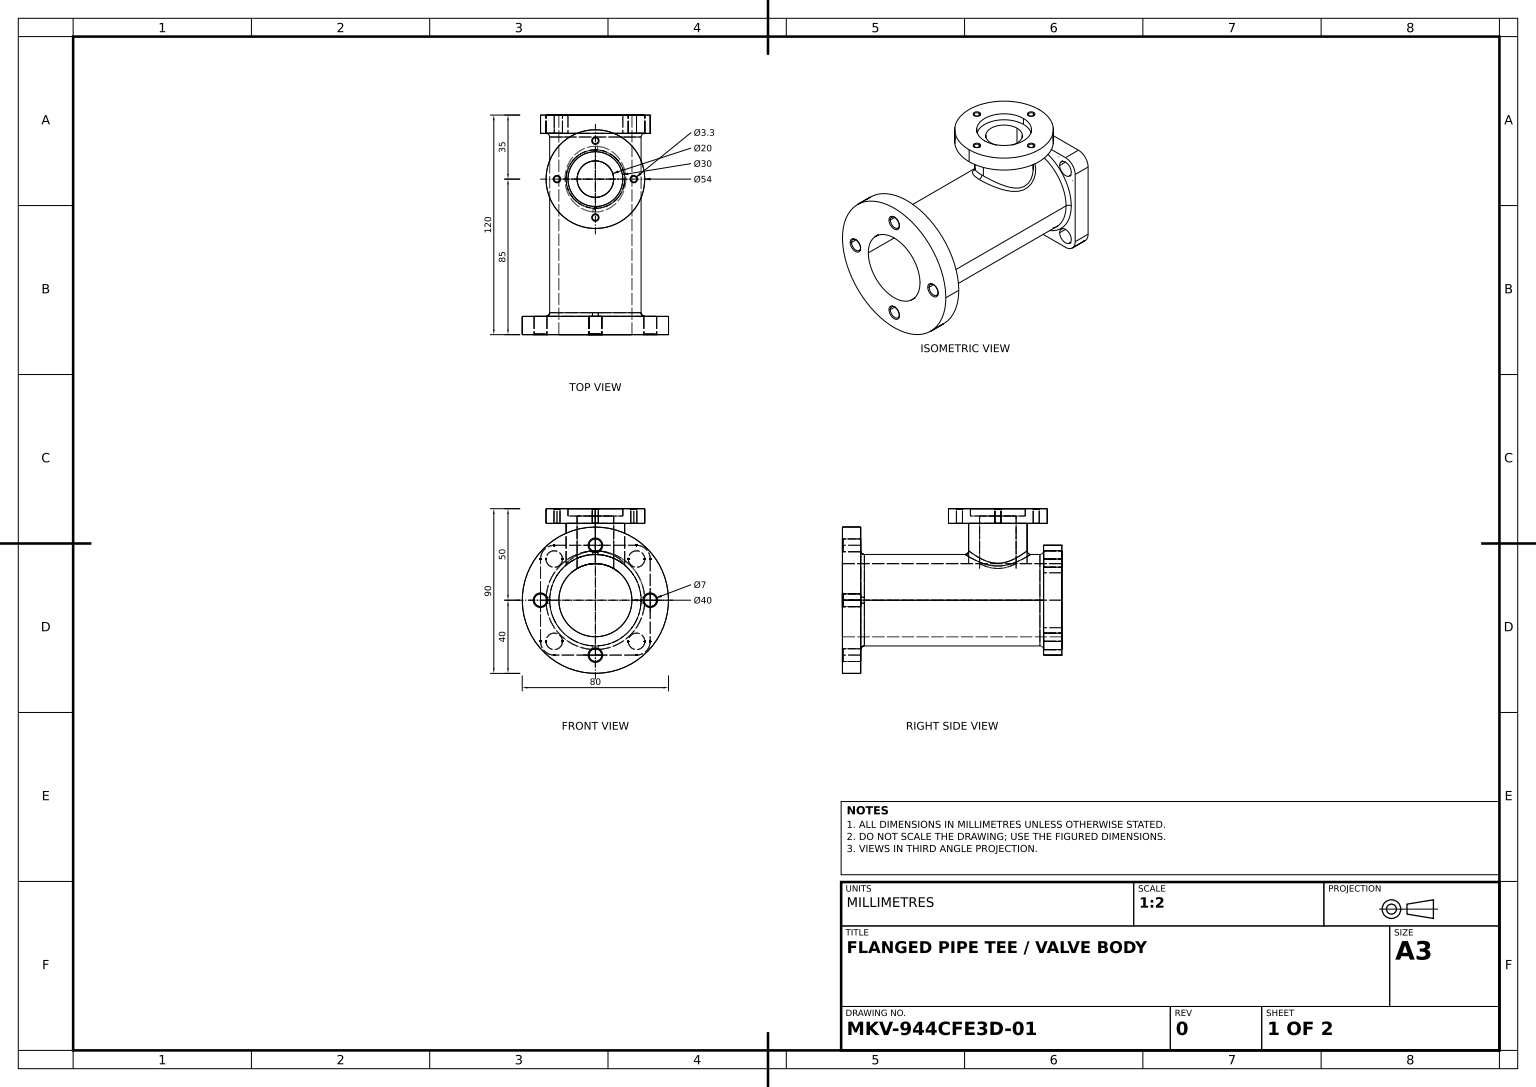
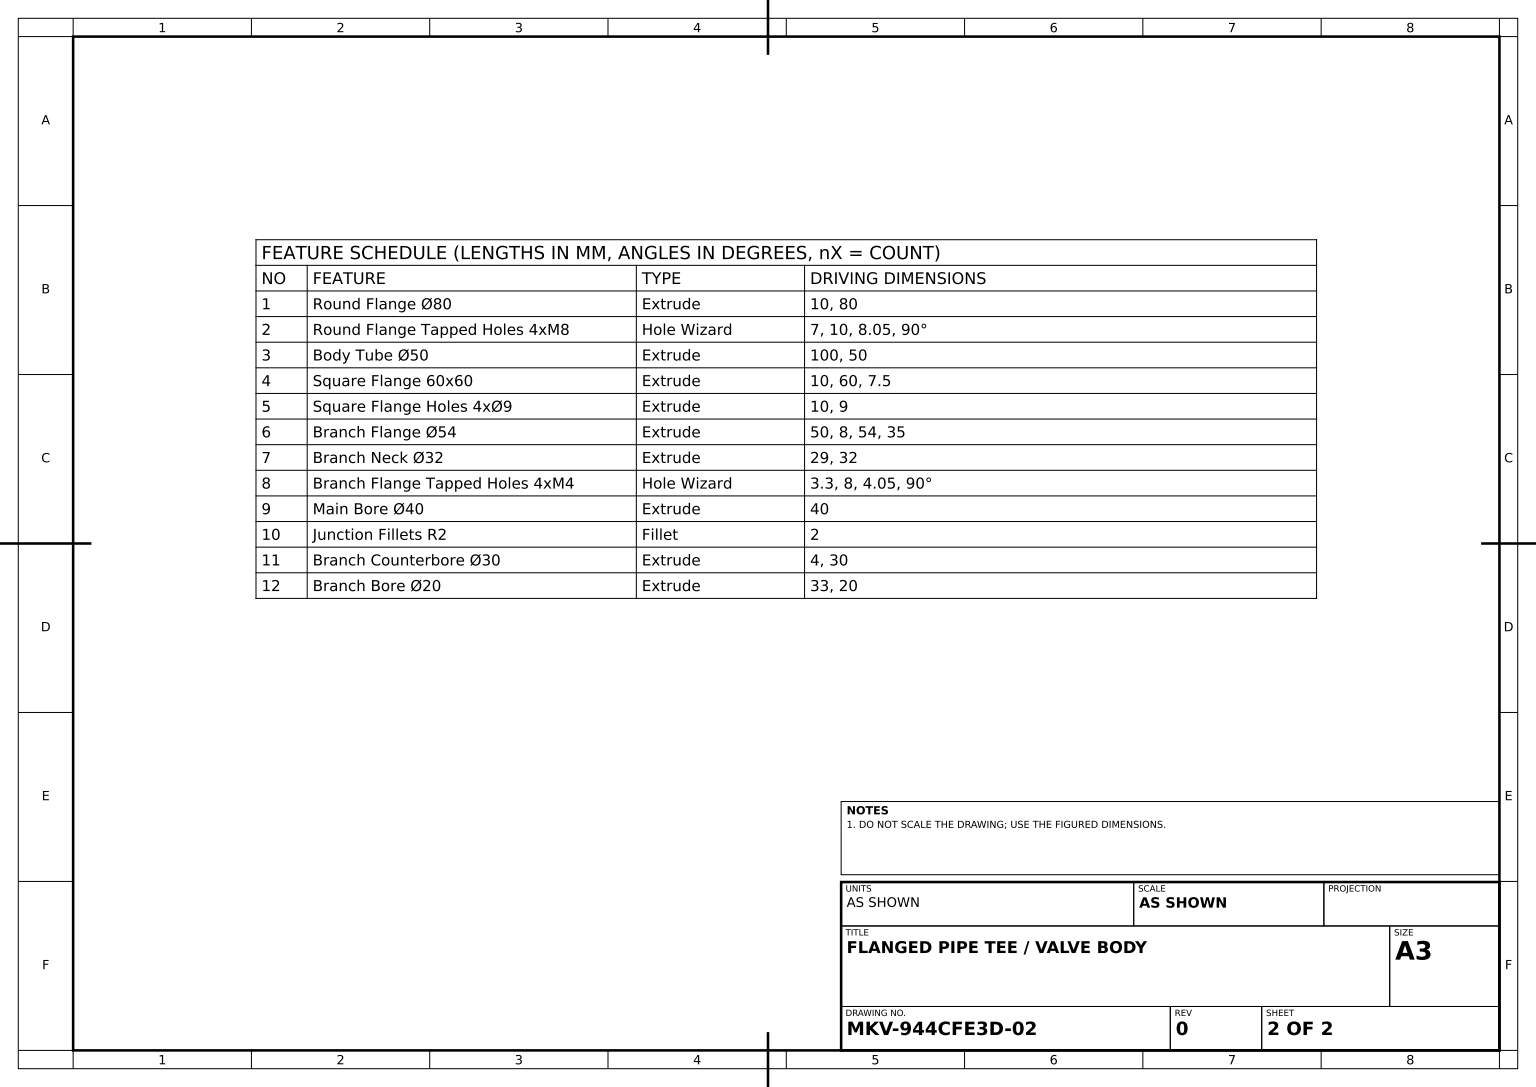
SolidWorks part; units mm, degrees
material "Plain Carbon Steel"
ref_plane "Front Plane" through (0, 0, 0) normal (0, 0, 1) x (1, 0, 0)
ref_plane "Top Plane" through (0, 0, 0) normal (0, 1, 0) x (1, 0, 0)
ref_plane "Right Plane" through (0, 0, 0) normal (1, 0, 0) x (0, 0, -1)
sketch "Round Flange Sketch" plane through (0, 0, 0) normal (0, 0, 1) x (1, 0, 0)
  circle A0 centre (0, 0) radius 40
  dimension "D1" = 80
extrude "Round Flange Ø80" add sketch "Round Flange Sketch" along normal blind 10
sketch "M8 Hole Positions Sketch" plane through (0, 0, 10) normal (0, 0, 1) x (1, 0, 0)
  line L0 (-40, 0) -> (40, 0) construction
  line L1 (0, 40) -> (0, -40) construction
  circle A0 centre (0, 0) radius 40 construction
  point P11 (-30, 0)
  point P12 (0, 30)
  point P13 (30, 0)
  point P14 (0, -30)
  dimension "D1" = 30
  dimension "D2" = 30
  dimension "D3" = 30
  dimension "D4" = 30
hole_wizard "Round Flange Tapped Holes 4xM8" positions "3DSketch4" profile "Sketch8" tap size "M8x1.0" standard "ANSI Metric" end condition through all
sketch3d "3DSketch4"
  point P0 (-30, 0, 10)
  point P3 (30, 0, 10)
  point P6 (0, 30, 10)
  point P9 (0, -30, 10)
sketch "Sketch8" plane through (-30, 0, 10) normal (1, 0, 0) x (0, -1, 0)
  line L0 (0, 0) -> (0, 10)
  line L1 (0, 10) -> (3.5, 10)
  line L2 (3.5, 10) -> (3.5, 0.525)
  line L3 (3.5, 0.525) -> (4.025, 0)
  line L5 (4.025, 0) -> (0, 0)
  line L6 (-3.5, 0.525) -> (-4.025, 0) construction
  line L11 (0, -6.35) -> (0, 107.95) construction
  dimension "Thru Tap Drill Dia." = 7
  dimension "Thru Tap Drill Depth" = 10
  dimension "Near C'Sink Dia." = 8.05
  dimension "Near C'Sink Angle" = 90
cosmetic thread "Hole Thread1" parameters "D2"=8
cosmetic thread "Hole Thread2" parameters "D2"=8
cosmetic thread "Hole Thread3" parameters "D2"=8
cosmetic thread "Hole Thread4" parameters "D2"=8
sketch "Body Tube Sketch" plane through (0, 0, 0) normal (0, 0, -1) x (-1, 0, 0)
  circle A0 centre (0, 0) radius 25
  dimension "D1" = 50
extrude "Body Tube Ø50" add sketch "Body Tube Sketch" along normal blind 100
sketch "Square Flange Sketch" plane through (0, 0, -100) normal (0, 0, -1) x (-1, 0, 0)
  line L1 (-22.5, -30) -> (22.5, -30)
  line L2 (-30, -22.5) -> (-30, 22.5)
  line L3 (-22.5, 30) -> (22.5, 30)
  line L4 (30, -22.5) -> (30, 22.5)
  line L5 (-30, -30) -> (30, 30) construction
  line L6 (-30, 30) -> (30, -30) construction
  arc A0 (-30, 22.5) -> (-22.5, 30) centre (-22.5, 22.5) cw
  arc A1 (-22.5, -30) -> (-30, -22.5) centre (-22.5, -22.5) cw
  arc A2 (22.5, -30) -> (30, -22.5) centre (22.5, -22.5) ccw
  arc A3 (22.5, 30) -> (30, 22.5) centre (22.5, 22.5) cw
  point P0 (0, 0)
  dimension "D3" = 7.5
  dimension "D4" = 7.5
  dimension "D1" = 60
  dimension "D2" = 60
extrude "Square Flange 60x60" add sketch "Square Flange Sketch" along normal blind 10
sketch "Square Flange Holes Sketch" plane through (0, 0, -110) normal (0, 0, -1) x (-1, 0, 0)
  circle A0 centre (22.5, 22.5) radius 4.5
  circle A1 centre (22.5, -22.5) radius 4.5
  circle A2 centre (-22.5, -22.5) radius 4.5
  circle A3 centre (-22.5, 22.5) radius 4.5
  dimension "D1" = 9
  dimension "D2" = 9
  dimension "D3" = 9
  dimension "D4" = 9
  dimension "D5" = 45
extrude "Square Flange Holes 4xØ9" cut sketch "Square Flange Holes Sketch" against normal blind 10
ref_plane "Plane1" through (0, 50, 0) normal (0, 1, 0) x (1, 0, 0)
sketch "Branch Flange Sketch" plane through (0, 50, 0) normal (0, 1, 0) x (1, 0, 0)
  line L0 (-22.5, 110) -> (22.5, 110) construction
  circle A0 centre (0, 75) radius 27
  dimension "D1" = 54
  dimension "D2" = 35
extrude "Branch Flange Ø54" add sketch "Branch Flange Sketch" against normal blind 8 separate body
sketch "Branch Neck Sketch" plane through (0, 42, 0) normal (0, -1, 0) x (1, 0, 0)
  circle A0 centre (0, -75) radius 16
  dimension "D1" = 32
extrude "Branch Neck Ø32" add sketch "Branch Neck Sketch" along normal blind 29
sketch "M4 Hole Positions Sketch" plane through (0, 50, 0) normal (0, 1, 0) x (1, 0, 0)
  circle A0 centre (0, 75) radius 21
  point P3 (0, 96)
  point P4 (21, 75)
  point P5 (0, 54)
  point P6 (-21, 75)
  dimension "D1" = 42
hole_wizard "Branch Flange Tapped Holes 4xM4" positions "3DSketch6" profile "Sketch17" tap size "M4x0.7" standard "ANSI Metric"
sketch3d "3DSketch6"
  point P0 (0, 50, -96)
  point P3 (-21, 50, -75)
  point P6 (0, 50, -54)
  point P9 (21, 50, -75)
sketch "Sketch17" plane through (0, 50, -96) normal (1, 0, 0) x (0, 0, 1)
  line L0 (0, 0) -> (0, 8)
  line L1 (0, 8) -> (1.65, 8)
  line L2 (1.65, 8) -> (1.65, 0.375)
  line L3 (1.65, 0.375) -> (2.025, 0)
  line L5 (2.025, 0) -> (0, 0)
  line L6 (-1.65, 0.375) -> (-2.025, 0) construction
  line L11 (0, -6.35) -> (0, 107.95) construction
  dimension "Thru Tap Drill Dia." = 3.3
  dimension "Thru Tap Drill Depth" = 8
  dimension "Near C'Sink Dia." = 4.05
  dimension "Near C'Sink Angle" = 90
cosmetic thread "Hole Thread9" parameters "D2"=4
cosmetic thread "Hole Thread10" parameters "D2"=4
cosmetic thread "Hole Thread11" parameters "D2"=4
cosmetic thread "Hole Thread12" parameters "D2"=4
sketch "Main Bore Sketch" plane through (0, 0, 10) normal (0, 0, 1) x (1, 0, 0)
  circle A0 centre (0, 0) radius 20
  dimension "D1" = 40
extrude "Main Bore Ø40" cut sketch "Main Bore Sketch" against normal through all
fillet "Junction Fillets R2" radius 2 3 edges at (-25, 0, -100) (-25, 0, 0) (-2.7646, 24.8467, -90.7593)
sketch "Branch Counterbore Sketch" plane through (0, 50, 0) normal (0, 1, 0) x (1, 0, 0)
  circle A0 centre (0, 75) radius 15
  dimension "D1" = 30
extrude "Branch Counterbore Ø30" cut sketch "Branch Counterbore Sketch" against normal blind 4
sketch "Branch Bore Sketch" plane through (0, 46, 0) normal (0, 1, 0) x (1, 0, 0)
  circle A0 centre (0, 75) radius 10
  dimension "D1" = 20
extrude "Branch Bore Ø20" cut sketch "Branch Bore Sketch" against normal blind 33
